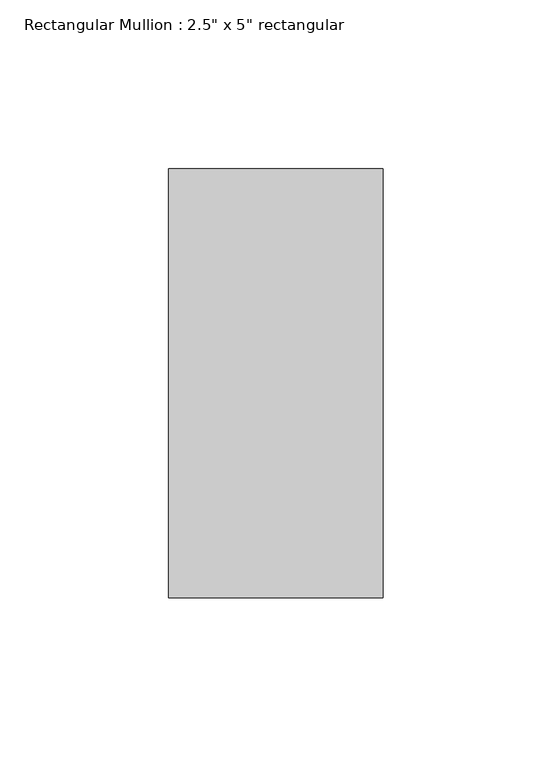
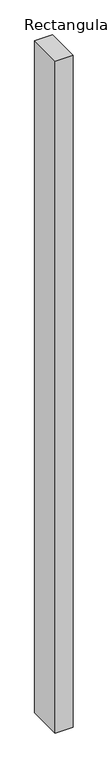
"""IFC4 building model written with IfcOpenShell, lengths in millimetres: member geometry."""

from ifc_helpers import new_model, si_unit, frame, origin, place, context, project, spatial, polyline, outline, extrude, source, transform, mapped, element, save


def member_bc34c253(model_context):
    return source(origin(), model_context, "Body", "SweptSolid", [
        extrude(outline(polyline([(31.75, 63.5), (31.75, -63.5), (-31.75, -63.5), (-31.75, 63.5), (31.75, 63.5)])), frame((0.0, 0.0, -2540.0), z_axis=(0.0, 0.0, 1.0), x_axis=(1.0, 0.0, 0.0)), (0.0, 0.0, 1.0), 2540.0),
    ])


if __name__ == "__main__":
    model = new_model("IFC4")
    model_context = context("Model", 3, world=origin())
    ifc_project = project(units=[si_unit("LENGTHUNIT", "METRE", prefix="MILLI")], contexts=[model_context])
    site = spatial("IfcSite", under=ifc_project)
    building = spatial("IfcBuilding", under=site)
    placement = place(None, origin())
    member_shape = member_bc34c253(model_context)
    element("IfcMember", 1, ObjectType="Rectangular Mullion : 2.5\" x 5\" rectangular", at=placement, inside=building, context=model_context, shape_type="MappedRepresentation", body=[
        mapped(member_shape, transform((0.0, 0.0, 0.0), x_axis=(1.0, 0.0, 0.0), y_axis=(0.0, 1.0, 0.0), z_axis=(0.0, 0.0, 1.0))),
    ])
    save(model, "model.ifc")

# Revit data of these elements
# Type "Rectangular Mullion : 2.5\" x 5\" rectangular"
#   built-in parameter 1007304 = 0.416667 (stored number, unit not read)
#   built-in parameter 1007301 = 0.104167 (stored number, unit not read)
#   built-in parameter 1007300 = 0.104167 (stored number, unit not read)
# Element 1 (IfcMember, "Rectangular Mullion : 2.5\" x 5\" rectangular")
#   Materials on its faces: "Aluminum"
# Materials
#   "Aluminum": class "Metal", colour RGB 247 247 247, transparency 0, Description = "Aluminum 6061", Cost = 0
